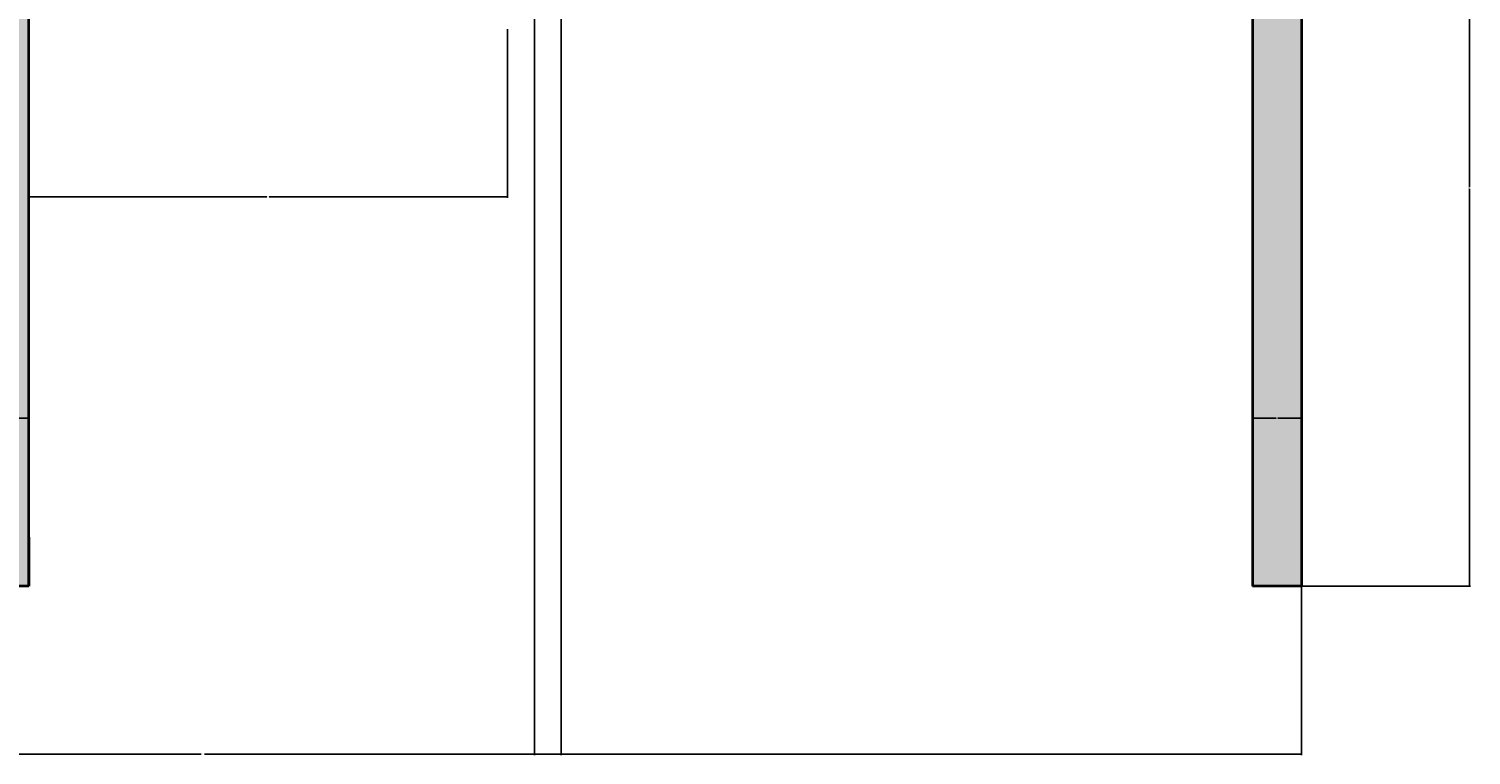
# Model space of a CAD drawing. Units: inches. Extents: x -30 to 437, y -29 to 647.
# Tile 5 of 15: x 172 to 437, y -29 to 105. Entities that reach past the tile are written whole.
import ezdxf

# ---------------------------------------------------------------- set-up
doc = ezdxf.new("R2010")
doc.units = ezdxf.units.IN
doc.header["$MEASUREMENT"] = 0
doc.layers.add('A-ANNO-DIMS', color=2, linetype='Continuous', lineweight=18)
doc.layers.add('A-WALL', color=7, linetype='Continuous', lineweight=35)
doc.layers.add('A-WALL-PATT', color=251, linetype='Continuous', lineweight=13, true_color=0x636466)
doc.styles.get("Standard").update_dxf_attribs({"font": 'arial.ttf'})
doc.dimstyles.get("Standard").update_dxf_attribs({"dimtxt": 0.18, "dimasz": 0.18, "dimexe": 0.18, "dimexo": 0.0625, "dimgap": 0.09, "dimtad": 0, "dimtih": 1, "dimtoh": 1, "dimdec": 4, "dimzin": 0, "dimdsep": 46, "dimtxsty": 'Standard', "dimcen": 0.09, "dimadec": 0, "dimazin": 0, "dimtfac": 1, "dimtdec": 4, "dimtofl": 0, "dimtmove": 0, "dimatfit": 3, "dimfxl": 1, "dimtolj": 1, "dimtzin": 0, "dimarcsym": 0})

# ---------------------------------------------------------------- blocks, each defined once
blk = doc.blocks.new('*D25')
at = {"layer": 'A-ANNO-DIMS', "color": 0, "lineweight": -2, "transparency": 16777216}
for p, q in [((1.67, 1.98), (1.67, -29.03)), ((405.67, 1.98), (405.67, -29.03)), ((1.85, -28.85), (203.38, -28.85)), ((405.49, -28.85), (203.97, -28.85))]:
    blk.add_line(p, q, dxfattribs=at)
at = {"layer": 'A-ANNO-DIMS', "color": 0, "transparency": 16777216}
for points in [[(1.85, -28.82), (1.85, -28.88), (1.67, -28.85)], [(405.49, -28.82), (405.49, -28.88), (405.67, -28.85)]]:
    blk.add_solid(points, dxfattribs=at)
at = {"layer": 'Defpoints', "color": 0, "transparency": 16777216}
for p in [(1.67, 2.05), (405.67, 2.05), (405.67, -28.85)]:
    blk.add_point(p, dxfattribs=at)
at = {"layer": 'A-ANNO-DIMS', "color": 0, "transparency": 16777216, "insert": (203.67, -28.85), "char_height": 0.18, "attachment_point": 5}
blk.add_mtext('\\A1;404', dxfattribs=at)
blk = doc.blocks.new('*D35')
at = {"layer": 'A-ANNO-DIMS', "color": 0, "lineweight": -2, "transparency": 16777216}
for p, q in [((1.67, 2.11), (1.67, 33.13)), ((1.85, 32.95), (86.39, 32.95)), ((171.49, 32.95), (86.95, 32.95)), ((171.67, 2.11), (171.67, 33.13))]:
    blk.add_line(p, q, dxfattribs=at)
at = {"layer": 'A-ANNO-DIMS', "color": 0, "transparency": 16777216}
for points in [[(1.85, 32.98), (1.85, 32.92), (1.67, 32.95)], [(171.49, 32.98), (171.49, 32.92), (171.67, 32.95)]]:
    blk.add_solid(points, dxfattribs=at)
at = {"layer": 'Defpoints', "color": 0, "transparency": 16777216}
for p in [(171.67, 32.95), (1.67, 2.05), (171.67, 2.05)]:
    blk.add_point(p, dxfattribs=at)
at = {"layer": 'A-ANNO-DIMS', "color": 0, "transparency": 16777216, "insert": (86.67, 32.95), "char_height": 0.18, "attachment_point": 5}
blk.add_mtext('\\A1;170', dxfattribs=at)
blk = doc.blocks.new('*D36')
at = {"layer": 'A-ANNO-DIMS', "color": 0, "lineweight": -2, "transparency": 16777216}
for p, q in [((171.67, 104.48), (171.67, 73.47)), ((259.67, 104.48), (259.67, 73.47)), ((171.85, 73.65), (215.45, 73.65)), ((259.49, 73.65), (215.89, 73.65))]:
    blk.add_line(p, q, dxfattribs=at)
at = {"layer": 'A-ANNO-DIMS', "color": 0, "transparency": 16777216}
for points in [[(171.85, 73.68), (171.85, 73.62), (171.67, 73.65)], [(259.49, 73.68), (259.49, 73.62), (259.67, 73.65)]]:
    blk.add_solid(points, dxfattribs=at)
at = {"layer": 'Defpoints', "color": 0, "transparency": 16777216}
for p in [(171.67, 104.55), (259.67, 104.55), (171.67, 73.65)]:
    blk.add_point(p, dxfattribs=at)
at = {"layer": 'A-ANNO-DIMS', "color": 0, "transparency": 16777216, "insert": (215.67, 73.65), "char_height": 0.18, "attachment_point": 5}
blk.add_mtext('\\A1;88', dxfattribs=at)
blk = doc.blocks.new('*D38')
at = {"layer": 'A-ANNO-DIMS', "color": 0, "lineweight": -2, "transparency": 16777216}
for p, q in [((396.67, 2.11), (396.67, 33.13)), ((396.85, 32.95), (401.02, 32.95)), ((405.49, 32.95), (401.32, 32.95)), ((405.67, 2.11), (405.67, 33.13))]:
    blk.add_line(p, q, dxfattribs=at)
at = {"layer": 'A-ANNO-DIMS', "color": 0, "transparency": 16777216}
for points in [[(396.85, 32.98), (396.85, 32.92), (396.67, 32.95)], [(405.49, 32.98), (405.49, 32.92), (405.67, 32.95)]]:
    blk.add_solid(points, dxfattribs=at)
at = {"layer": 'Defpoints', "color": 0, "transparency": 16777216}
for p in [(405.67, 32.95), (396.67, 2.05), (405.67, 2.05)]:
    blk.add_point(p, dxfattribs=at)
at = {"layer": 'A-ANNO-DIMS', "color": 0, "transparency": 16777216, "insert": (401.17, 32.95), "char_height": 0.18, "attachment_point": 5}
blk.add_mtext('\\A1;9', dxfattribs=at)
blk = doc.blocks.new('*D39')
at = {"layer": 'A-ANNO-DIMS', "color": 0, "lineweight": -2, "transparency": 16777216}
for p, q in [((396.74, 148.55), (436.75, 148.55)), ((436.57, 148.37), (436.57, 75.48)), ((436.57, 2.23), (436.57, 75.12)), ((396.74, 2.05), (436.75, 2.05))]:
    blk.add_line(p, q, dxfattribs=at)
at = {"layer": 'A-ANNO-DIMS', "color": 0, "transparency": 16777216}
for points in [[(436.54, 148.37), (436.6, 148.37), (436.57, 148.55)], [(436.54, 2.23), (436.6, 2.23), (436.57, 2.05)]]:
    blk.add_solid(points, dxfattribs=at)
at = {"layer": 'Defpoints', "color": 0, "transparency": 16777216}
for p in [(396.67, 148.55), (436.57, 148.55), (396.67, 2.05)]:
    blk.add_point(p, dxfattribs=at)
at = {"layer": 'A-ANNO-DIMS', "color": 0, "transparency": 16777216, "insert": (436.57, 75.3), "char_height": 0.18, "attachment_point": 5}
blk.add_mtext('\\A1;146.5', dxfattribs=at)
blk = doc.blocks.new('*D56')
at = {"layer": 'A-ANNO-DIMS', "color": 0, "lineweight": -2, "transparency": 16777216}
for p, q in [((269.54, 160.3), (269.54, -29.03)), ((264.67, 153.48), (264.67, -29.03)), ((264.85, -28.85), (266.78, -28.85)), ((269.36, -28.85), (267.44, -28.85))]:
    blk.add_line(p, q, dxfattribs=at)
at = {"layer": 'A-ANNO-DIMS', "color": 0, "transparency": 16777216}
for points in [[(264.85, -28.82), (264.85, -28.88), (264.67, -28.85)], [(269.36, -28.82), (269.36, -28.88), (269.54, -28.85)]]:
    blk.add_solid(points, dxfattribs=at)
at = {"layer": 'Defpoints', "color": 0, "transparency": 16777216}
for p in [(269.54, 160.37), (264.67, 153.55), (269.54, -28.85)]:
    blk.add_point(p, dxfattribs=at)
at = {"layer": 'A-ANNO-DIMS', "color": 0, "transparency": 16777216, "insert": (267.11, -28.85), "char_height": 0.18, "attachment_point": 5}
blk.add_mtext('\\A1;4.87', dxfattribs=at)

msp = doc.modelspace()

# ---------------------------------------------------------------- hatches: boundary and pattern name
at = {"layer": 'A-WALL-PATT'}
h = msp.add_hatch(color=256, dxfattribs=at)
h.dxf.hatch_style = 1
h.paths.add_polyline_path([(393.6054, 183.2352), (369.6054, 183.2352), (369.6054, 213.2352), (393.6054, 213.2352), (393.6054, 207.2352), (394.6054, 207.2352), (394.6054, 211.2352), (395.6054, 211.2352), (395.6054, 185.2352), (394.6054, 185.2352), (394.6054, 189.2352), (393.6054, 189.2352)], flags=0)
h.paths.add_polyline_path([(384.6054, 189.2352, -1), (390.6054, 189.2352, -1)], flags=0)
h.paths.add_polyline_path([(385.6054, 189.2352, -1), (389.6054, 189.2352, -1)], flags=0)
h.paths.add_polyline_path([(374.6054, 189.2352, -1), (382.6054, 189.2352, -1)], flags=0)
h.paths.add_polyline_path([(386.6054, 189.2352, -1), (388.6054, 189.2352, -1)], flags=0)
h.paths.add_polyline_path([(375.6054, 189.2352, -1), (381.6054, 189.2352, -1)], flags=0)
h.paths.add_polyline_path([(376.6054, 189.2352, -1), (380.6054, 189.2352, -1)], flags=0)
h.paths.add_polyline_path([(377.6054, 189.2352, -1), (379.6054, 189.2352, -1)], flags=0)
h.paths.add_polyline_path([(390.6054, 195.2352), (374.6054, 195.2352), (374.6054, 201.2352), (390.6054, 201.2352)], flags=0)
h.paths.add_polyline_path([(389.6054, 196.2352), (375.6054, 196.2352), (375.6054, 200.2352), (389.6054, 200.2352)], flags=0)
h.paths.add_polyline_path([(383.6054, 207.2352, -1), (391.6054, 207.2352, -1)], flags=0)
h.paths.add_polyline_path([(384.6054, 207.2352, -1), (390.6054, 207.2352, -1)], flags=0)
h.paths.add_polyline_path([(385.6054, 207.2352, -1), (389.6054, 207.2352, -1)], flags=0)
h.paths.add_polyline_path([(386.6054, 207.2352, -1), (388.6054, 207.2352, -1)], flags=0)
h.paths.add_polyline_path([(375.6054, 207.2352, -1), (381.6054, 207.2352, -1)], flags=0)
h.paths.add_polyline_path([(376.6054, 207.2352, -1), (380.6054, 207.2352, -1)], flags=0)
h.paths.add_polyline_path([(377.6054, 207.2352, -1), (379.6054, 207.2352, -1)], flags=0)
h.paths.add_polyline_path([(305.5437, 160.3663, -0.41421356), (304.0437, 158.8663), (271.0437, 158.8663, -0.41421356), (269.5437, 160.3663), (269.5437, 178.3663, -0.41421356), (271.0437, 179.8663), (304.0437, 179.8663, -0.41421356), (305.5437, 178.3663)], flags=0)
h.paths.add_polyline_path([(304.0437, 165.3663, -0.41421356), (303.0437, 164.3663), (289.2937, 164.3663, -0.41421356), (288.2937, 165.3663), (288.2937, 177.3663, -0.41421356), (289.2937, 178.3663), (303.0437, 178.3663, -0.41421356), (304.0437, 177.3663)], flags=0)
h.paths.add_polyline_path([(296.5437, 171.3663, -1), (295.5437, 171.3663, -1)], flags=0)
h.paths.add_polyline_path([(286.7937, 165.3663, -0.41421356), (285.7937, 164.3663), (272.0437, 164.3663, -0.41421356), (271.0437, 165.3663), (271.0437, 177.3663, -0.41421356), (272.0437, 178.3663), (285.7937, 178.3663, -0.41421356), (286.7937, 177.3663)], flags=0)
h.paths.add_polyline_path([(279.5437, 171.3663, -1), (278.5437, 171.3663, -1)], flags=0)
h.paths.add_polyline_path([(360.6737, 290.5474), (360.6737, 300.5474), (396.6737, 300.5474), (396.6737, 290.5474)], flags=0)
h.paths.add_polyline_path([(259.6737, 124.5474), (259.6737, 114.5474), (171.6737, 114.5474), (171.6737, 124.5474)], flags=0)
h.paths.add_polyline_path([(288.0737, 215.3705), (286.7097, 214.583), (268.7097, 245.7599), (270.0737, 246.5474)], flags=0)
h.paths.add_polyline_path([(259.6737, 168.5474), (256.6737, 168.5474), (256.6737, 173.5474), (256.6737, 179.0224), (255.8753, 177.6395), (224.2956, 195.872, 0.12053744), (220.1737, 179.0224, 0.12053744), (216.0518, 195.872), (184.4721, 177.6395), (183.6737, 179.0224), (215.2836, 197.2724), (216.0821, 195.8895), (216.0518, 195.872, -0.12053744), (220.1737, 179.0224, -0.12053744), (224.2956, 195.872), (224.2653, 195.8895), (225.0638, 197.2724), (256.6737, 179.0224), (256.6737, 173.5474), (259.6737, 173.5474)], flags=0)
h.paths.add_polyline_path([(386.7943, 325.4601), (372.6871, 325.4601), (372.6871, 339.5673), (386.7943, 339.5673)], flags=0)
h.paths.add_polyline_path([(359.5875, 343.7429), (357.7905, 343.7429), (357.7905, 327.9179), (359.3933, 327.9179, 0.41420885), (361.5302, 330.0549), (361.5302, 341.8434, 0.41436161)], flags=0)
h.paths.add_polyline_path([(341.7887, 323.1235, -0.11921667), (340.7839, 323.1235)], flags=0)
h.paths.add_polyline_path([(379.6332, 328.8632), (379.6332, 332.2699), (376.0992, 332.2699, 0.39427733)], flags=0)
h.paths.add_polyline_path([(375.5299, 332.459, -1), (383.8511, 332.459, -1)], flags=0)
h.paths.add_polyline_path([(388.9363, 344.7425), (372.5309, 344.7425, -0.41421356), (370.394, 346.8794), (370.394, 347.5594, -0.39085173), (372.3472, 349.7005, -0.43951011), (370.394, 351.4933), (370.394, 365.1894, -0.40305452), (372.2191, 367.1298, -0.41839453), (370.394, 368.9291), (370.394, 382.6251, -0.40885826), (372.2519, 384.5722, -0.42377324), (370.394, 386.3707), (370.394, 400.0667, -0.38660687), (372.1327, 402.0094), (372.531, 402.0094, -0.41421834), (370.394, 404.1464), (370.394, 404.7778, -0.41420891), (372.5309, 406.9147), (388.9363, 406.9147, -0.41421821), (391.0733, 404.7778), (391.0733, 346.8794, -0.41421356)], flags=0)
edge = h.paths.add_edge_path(flags=0)
edge.add_spline(control_points=[(349.3585, 363.204), (349.0859, 363.204), (348.8133, 363.2227), (348.2712, 363.2973), (348.0016, 363.3531), (347.3533, 363.5328), (346.9776, 363.6755), (346.2445, 364.0308), (345.887, 364.2432), (345.1953, 364.7329), (344.8611, 365.0101), (344.2197, 365.6237), (343.9125, 365.9603), (343.211, 366.8336), (342.8313, 367.3965), (342.1401, 368.6117), (341.8286, 369.2641), (341.2807, 370.64), (341.0443, 371.3636), (340.6522, 372.8619), (340.4964, 373.6367), (340.2695, 375.2158), (340.1983, 376.0203), (340.142, 377.6365), (340.157, 378.4483), (340.2729, 380.0567), (340.3738, 380.8533), (340.6589, 382.4093), (340.8432, 383.1686), (341.2906, 384.629), (341.5538, 385.3301), (342.1531, 386.6544), (342.4891, 387.2776), (343.2266, 388.4288), (343.6281, 388.9567), (344.4879, 389.9012), (344.9463, 390.3178), (345.7981, 390.9428), (346.182, 391.1771), (346.9712, 391.5648), (347.3766, 391.7182), (348.2004, 391.9387), (348.6189, 392.0058), (349.4588, 392.0508), (349.8801, 392.0288), (350.7146, 391.8966), (351.1278, 391.7865), (351.9366, 391.4822), (352.3323, 391.2882), (353.0989, 390.8223), (353.4699, 390.5504), (354.1819, 389.9355), (354.5229, 389.5924), (355.1706, 388.8418), (355.4772, 388.4343), (356.1315, 387.4422), (356.4671, 386.8397), (357.0692, 385.5581), (357.3356, 384.879), (357.7933, 383.4624), (357.9846, 382.725), (358.2875, 381.2112), (358.3992, 380.4349), (358.5404, 378.8643), (358.5699, 378.0699), (358.546, 376.4841), (358.4926, 375.6928), (358.3042, 374.1343), (358.1692, 373.3672), (357.8207, 371.8774), (357.6072, 371.1549), (357.1067, 369.7735), (356.8196, 369.1148), (356.1782, 367.8787), (355.8238, 367.3013), (355.0551, 366.244), (354.6408, 365.7641), (353.7607, 364.9161), (353.2948, 364.5481), (352.445, 364.0149), (352.0701, 363.822), (351.3034, 363.5117), (350.9116, 363.3943), (350.1325, 363.2418), (349.7455, 363.204), (349.3585, 363.204)], knot_values=[3.14159265, 3.14159265, 3.14159265, 3.14159265, 3.22691715, 3.22691715, 3.31224165, 3.31224165, 3.43426671, 3.43426671, 3.55629177, 3.55629177, 3.67831683, 3.67831683, 3.8003419, 3.8003419, 3.97157384, 3.97157384, 4.14280577, 4.14280577, 4.31403771, 4.31403771, 4.48526965, 4.48526965, 4.65650159, 4.65650159, 4.82773353, 4.82773353, 4.99896547, 4.99896547, 5.1701974, 5.1701974, 5.34142934, 5.34142934, 5.51266128, 5.51266128, 5.68389322, 5.68389322, 5.85512516, 5.85512516, 5.98669107, 5.98669107, 6.11825699, 6.11825699, 6.24982291, 6.24982291, 6.38138882, 6.38138882, 6.51295474, 6.51295474, 6.64452065, 6.64452065, 6.77608657, 6.77608657, 6.90765249, 6.90765249, 7.0392184, 7.0392184, 7.20701563, 7.20701563, 7.37481286, 7.37481286, 7.54261009, 7.54261009, 7.71040732, 7.71040732, 7.87820455, 7.87820455, 8.04600178, 8.04600178, 8.21379901, 8.21379901, 8.38159624, 8.38159624, 8.54939347, 8.54939347, 8.7171907, 8.7171907, 8.88498794, 8.88498794, 9.05278517, 9.05278517, 9.17820699, 9.17820699, 9.30362881, 9.30362881, 9.42477796, 9.42477796, 9.42477796, 9.42477796], degree=3, periodic=0)
edge.add_line((341.1696, 384.3006), (341.2012, 384.2808))
edge = h.paths.add_edge_path(flags=0)
edge.add_line((344.3353, 388.7801), (344.317, 388.7915))
edge.add_ellipse((349.3585, 377.6204), major_axis=(0, -13.7895), ratio=0.62186025, start_angle=-244.867444, end_angle=-124.769923)
h.paths.add_polyline_path([(163.6737, 163.1474), (132.4968, 145.1474), (131.7093, 146.5114), (162.8862, 164.5114)], flags=0)
h.paths.add_polyline_path([(366.4355, 409.0896, -0.41423669), (364.2985, 406.9525, -0.4913499), (361.5302, 408.8973), (361.5302, 420.6405, 0.41421356), (359.3932, 422.7775), (357.7905, 422.7775), (357.7905, 406.9525), (359.6317, 406.9525, 0.42741026), (361.5332, 408.9757, 0.39869469), (363.6672, 406.9525, 0.51958103), (366.4355, 409.0895)], flags=0)
h.paths.add_polyline_path([(386.7943, 410.9671), (372.6871, 410.9671), (372.6871, 425.0742), (386.7943, 425.0742)], flags=0)
h.paths.add_polyline_path([(379.6332, 414.3701), (379.6332, 417.7768), (376.0992, 417.7768, 0.39427733)], flags=0)
h.paths.add_polyline_path([(375.5299, 417.966, -1), (383.8511, 417.966, -1)], flags=0)
h.paths.add_polyline_path([(150.0377, 351.583), (148.6737, 352.3705), (166.6737, 383.5474), (168.0377, 382.7599)], flags=0)
h.paths.add_polyline_path([(91.6737, 234.1974), (66.559, 219.6974), (65.9246, 220.7962), (91.0393, 235.2962)], flags=0)
h.paths.add_polyline_path([(255.4612, 443.5834), (254.6737, 444.9474), (285.8506, 462.9474), (286.6381, 461.5834)], flags=0)
h.paths.add_polyline_path([(176.2737, 394.5474), (158.2737, 425.7243), (159.6377, 426.5118), (177.6377, 395.3349)], flags=0)
h.paths.add_polyline_path([(243.6737, 439.5474), (243.0393, 438.4486), (217.9246, 452.9486), (218.559, 454.0474)], flags=0)
h.paths.add_polyline_path([(38.1264, 269.8429), (40.2408, 269.8429), (40.2408, 270.3508), (38.1264, 270.3508)], flags=0)
h.paths.add_polyline_path([(75.7157, 289.9439), (40.2408, 289.9439), (38.1264, 289.6524), (40.2408, 289.6524)], flags=0)
h.paths.add_polyline_path([(75.7157, 270.0846), (77.6447, 270.0846), (77.6697, 270.1626), (75.7175, 270.1626)], flags=0)
h.paths.add_polyline_path([(80.5373, 293.3002), (33.0467, 293.3002), (13.5054, 293.3002), (13.5054, 351.9244), (29.7898, 351.9244), (80.5373, 351.9244)], flags=0)
h.paths.add_polyline_path([(46.0261, 212.466, -0.50131678), (27.1651, 207.5106), (21.165, 209.5107), (21.165, 206.5107), (22.665, 206.5107), (22.665, 203.5107), (21.165, 203.5107), (21.165, 203.0107), (13.165, 203.0107), (13.165, 224.0107), (21.165, 224.0107), (21.165, 217.5107), (27.1649, 219.5106, -0.50132349), (46.0261, 214.5554, -0.13289091)], flags=0)
h.paths.add_polyline_path([(44.688, 211.8666, -0.48007965), (27.165, 209.5107), (27.165, 217.5107, -0.4800795), (44.688, 215.1547, -0.21500378)], flags=0)
h.paths.add_polyline_path([(19.415, 204.0107), (15.165, 204.0107, -0.41421356), (14.165, 204.7607), (14.165, 222.0107, -0.41421356), (14.915, 223.0107), (19.165, 223.0107, -0.41421356), (20.165, 222.2607), (20.165, 205.0107, -0.41421356)], flags=0)
h.paths.add_polyline_path([(32.7608, 269.0719), (31.8439, 269.0719), (31.8439, 268.6134), (13.5054, 268.6134), (13.5054, 291.5366), (31.8439, 291.5366), (32.7608, 291.0781), (32.7608, 280.9919, -1), (32.7608, 279.1581)], flags=0)
h.paths.add_polyline_path([(40.2408, 360.1436), (38.1264, 360.1436), (38.1264, 359.6357), (40.2408, 359.6357)], flags=0)
h.paths.add_polyline_path([(75.7157, 355.2807), (40.2408, 355.2807), (38.1264, 355.5722), (40.2408, 355.5722), (40.2408, 355.2807), (75.7157, 355.2807), (75.7157, 375.5982), (40.2408, 375.5982), (38.1264, 375.3817), (40.2408, 375.3817), (40.2408, 375.5982), (75.7157, 375.5982), (77.9733, 375.062), (75.7175, 375.062), (75.7175, 374.554)], flags=0)
h.paths.add_polyline_path([(42.8174, 299.814, 0.13867074), (34.1602, 294.603), (14.8081, 294.603), (14.8081, 350.6216), (29.8539, 350.6216, 0.09822056)], flags=0)
h.paths.add_polyline_path([(15.8636, 276.7781, -0.30640166), (20.3757, 283.4499), (20.3483, 290.6726), (31.4014, 290.7146), (31.4309, 282.9124), (26.8287, 282.895, -0.26006276), (30.241, 276.7781, -1)], flags=0)
h.paths.add_polyline_path([(26.1332, 276.7781), (23.0523, 273.6972), (19.9714, 276.7781), (23.0523, 279.8589), (23.0523, 283.9209), (21.3493, 283.9145), (20.7006, 283.5219), (20.6907, 286.1226), (23.2914, 286.1325), (25.8936, 285.7522), (27.1939, 285.7572), (28.4928, 286.1522), (31.0935, 286.1621), (31.0918, 286.6172), (25.6303, 286.5965), (25.616, 290.3675), (31.0775, 290.3882), (31.0918, 286.6172), (31.1034, 283.5614), (28.5027, 283.5515), (25.9005, 283.9317), (23.0523, 283.9209), (23.0523, 279.8589)], flags=0)
h.paths.add_polyline_path([(24.0793, 276.7781, -1), (22.0253, 276.7781, -1)], flags=0)
h.paths.add_polyline_path([(35.7687, 302.2895, -0.41421356), (35.2283, 301.2726), (22.2164, 297.2909, -0.41421356), (21.1995, 297.8313), (15.7317, 315.6996, -0.41421356), (16.2721, 316.7165), (18.8554, 317.507), (15.3721, 328.8904, -0.41421356), (15.9125, 329.9073), (28.9244, 333.889, -0.41421356), (29.9414, 333.3486), (35.4091, 315.4802, -0.41421356), (34.8687, 314.4633), (32.2854, 313.6728)], flags=0)
h.paths.add_polyline_path([(361.3728, 532.6207), (302.7487, 532.6207), (302.7487, 580.1113), (302.7487, 599.6527), (361.3728, 599.6527), (361.3728, 583.3682)], flags=0)
h.paths.add_polyline_path([(370.1, 575.0316), (370.1, 572.9172), (370.6079, 572.9172), (370.6079, 575.0316)], flags=0)
h.paths.add_polyline_path([(385.0466, 537.4423), (385.0466, 572.9172), (384.8302, 575.0316), (384.8302, 572.9172)], flags=0)
h.paths.add_polyline_path([(384.5104, 535.3262), (384.5104, 537.4406), (384.0025, 537.4406), (364.7291, 537.4423), (364.7291, 572.9172), (365.0206, 575.0316), (365.0206, 572.9172), (364.7291, 572.9172), (364.7291, 537.4423), (384.5884, 537.4423), (384.5884, 535.5133)], flags=0)
h.paths.add_polyline_path([(384.5884, 535.5133), (383.4945, 535.164), (383.4945, 537.4406), (382.9866, 535.3262), (382.9866, 537.4406), (383.4945, 535.3262), (383.4945, 537.4406), (384.5884, 537.4406)], flags=0)
h.paths.add_polyline_path([(23.874, 286.8174), (21.0132, 286.8065), (21.0004, 290.1875), (23.8612, 290.1983)], flags=0)
h.paths.add_polyline_path([(242.9824, 511.1667), (234.9824, 511.1667), (234.9824, 517.6667), (228.9825, 515.6667, -0.50132349), (210.1213, 520.622, -0.13289091), (210.1213, 522.7114, -0.50131678), (228.9823, 527.6667), (234.9824, 525.6667), (234.9824, 528.6667), (233.4824, 528.6667), (233.4824, 531.6667), (234.9824, 531.6667), (234.9824, 532.1667), (242.9824, 532.1667)], flags=0)
h.paths.add_polyline_path([(236.9824, 512.1667, -0.41421356), (235.9824, 512.9167), (235.9824, 530.1667, -0.41421356), (236.7324, 531.1667), (240.9824, 531.1667, -0.41421356), (241.9824, 530.4167), (241.9824, 513.1667, -0.41421356), (241.2324, 512.1667)], flags=0)
h.paths.add_polyline_path([(279.533, 537.4423), (279.533, 535.5133), (279.6111, 535.4884), (279.6111, 537.4406)], flags=0)
h.paths.add_polyline_path([(279.2913, 575.0316), (279.2913, 572.9172), (279.7992, 572.9172), (279.7992, 575.0316)], flags=0)
h.paths.add_polyline_path([(211.4594, 520.0227, -0.21500378), (211.4594, 523.3107, -0.48007965), (228.9824, 525.6667), (228.9824, 517.6667, -0.4800795)], flags=0)
h.paths.add_polyline_path([(32.7627, 354.1465), (31.8457, 354.1465), (31.8457, 353.688), (13.5054, 353.688), (13.5054, 376.6134), (31.8457, 376.6134), (32.7627, 376.1549), (32.7627, 366.0677, -1), (32.7627, 364.2337)], flags=0)
h.paths.add_polyline_path([(15.9446, 365.1507, -1), (30.3234, 365.1507, -1)], flags=0)
h.paths.add_polyline_path([(41.213, 428.467), (43.3274, 428.467), (43.3274, 428.9749), (41.213, 428.9749)], flags=0)
h.paths.add_polyline_path([(78.8022, 448.568), (43.3274, 448.568), (41.213, 448.2765), (43.3274, 448.2765)], flags=0)
h.paths.add_polyline_path([(78.8022, 428.7087), (80.7313, 428.7087), (80.7562, 428.7868), (78.804, 428.7868)], flags=0)
h.paths.add_polyline_path([(26.2152, 365.1507), (23.134, 362.0696), (20.0529, 365.1507), (23.134, 368.2319)], flags=0)
h.paths.add_polyline_path([(24.1611, 365.1507, -1), (22.107, 365.1507, -1)], flags=0)
h.paths.add_polyline_path([(309.2625, 570.3406, 0.13867074), (304.0514, 578.9978), (304.0514, 598.3499), (360.07, 598.3499), (360.07, 583.3041, 0.09822056)], flags=0)
h.paths.add_polyline_path([(246.6737, 552.5474), (129.6737, 552.5474), (129.6737, 606.5474), (246.6737, 606.5474)], flags=16)
h.paths.add_polyline_path([(373.6822, 580.3953), (363.595, 580.3953), (363.595, 581.3123), (363.1365, 581.3123), (363.1365, 599.6527), (386.0619, 599.6527), (386.0619, 581.3123), (385.6034, 580.3953), (375.5162, 580.3953, -1)], flags=0)
h.paths.add_polyline_path([(83.6239, 451.9244), (36.1333, 451.9244), (16.5919, 451.9244), (16.5919, 510.5485), (32.8764, 510.5485), (83.6239, 510.5485)], flags=0)
h.paths.add_polyline_path([(367.4098, 590.024, -1), (381.7886, 590.024, -1)], flags=0)
h.paths.add_polyline_path([(374.5992, 586.9428), (371.518, 590.024), (374.5992, 593.1052), (377.6803, 590.024)], flags=0)
h.paths.add_polyline_path([(373.5721, 590.024, -1), (375.6262, 590.024, -1)], flags=0)
h.paths.add_polyline_path([(324.9287, 577.7489, -0.41421356), (323.9118, 578.2893), (323.1212, 580.8726), (311.7379, 577.3893, -0.41421356), (310.721, 577.9297), (306.7393, 590.9416, -0.41421356), (307.2797, 591.9585), (325.1481, 597.4263, -0.41421356), (326.165, 596.8859), (326.9555, 594.3026), (338.3388, 597.7859, -0.41421356), (339.3557, 597.2455), (343.3374, 584.2336, -0.41421356), (342.797, 583.2167)], flags=0)
h.paths.add_polyline_path([(300.5265, 580.3972), (290.4404, 580.3972, -1), (288.6065, 580.3972), (278.5203, 580.3972), (278.5203, 581.3142), (278.0619, 581.3142), (278.0619, 599.6527), (300.985, 599.6527), (300.985, 581.3142)], flags=0)
h.paths.add_polyline_path([(300.163, 581.7567), (292.3609, 581.7271), (292.3434, 586.3294, -0.75567924), (279.0378, 590.1057, -0.82536731), (292.8983, 592.7823), (300.1211, 592.8097)], flags=0)
h.paths.add_polyline_path([(299.8367, 582.0805), (296.0656, 582.0662), (293.0098, 582.0546), (292.9999, 584.6553), (293.3802, 587.2575), (293.3694, 590.1057), (289.3074, 590.1057), (286.2265, 587.0248), (283.1456, 590.1057), (286.2265, 593.1866), (289.3074, 590.1057), (293.3694, 590.1057), (293.3629, 591.8088), (292.9703, 592.4575), (295.5711, 592.4673), (295.5809, 589.8666), (295.2007, 587.2644), (295.2056, 585.9641), (295.6006, 584.6652), (295.6105, 582.0645), (296.0656, 582.0662), (296.0449, 587.5277), (299.8159, 587.542)], flags=0)
h.paths.add_polyline_path([(285.1995, 590.1057, -1), (287.2535, 590.1057, -1)], flags=0)
h.paths.add_polyline_path([(299.6467, 589.2969), (296.2658, 589.284), (296.255, 592.1448), (299.6359, 592.1576)], flags=0)
h.paths.add_polyline_path([(35.8473, 427.696), (34.9304, 427.696), (34.9304, 427.2376), (16.5919, 427.2376), (16.5919, 450.1607), (34.9304, 450.1607), (35.8473, 449.7022), (35.8473, 439.6161, -1), (35.8473, 437.7822)], flags=0)
h.paths.add_polyline_path([(18.9502, 435.4022, -0.30640166), (23.4623, 442.074), (23.4349, 449.2968), (34.4879, 449.3387), (34.5175, 441.5366), (29.9152, 441.5191, -0.26006276), (33.3275, 435.4022, -1)], flags=0)
h.paths.add_polyline_path([(29.2197, 435.4022), (26.1389, 432.3213), (23.058, 435.4022), (26.1389, 438.4831), (26.1389, 442.5451), (24.4358, 442.5386), (23.7871, 442.1461), (23.7772, 444.7468), (26.378, 444.7566), (28.9801, 444.3764), (30.2805, 444.3813), (31.5794, 444.7764), (34.1801, 444.7862), (34.1784, 445.2413), (28.7169, 445.2206), (28.7026, 448.9917), (34.164, 449.0124), (34.1784, 445.2413), (34.1899, 442.1855), (31.5892, 442.1756), (28.987, 442.5559), (26.1389, 442.5451), (26.1389, 438.4831)], flags=0)
h.paths.add_polyline_path([(27.1658, 435.4022, -1), (25.1119, 435.4022, -1)], flags=0)
h.paths.add_polyline_path([(45.904, 458.4382, 0.13867074), (37.2467, 453.2271), (17.8947, 453.2271), (17.8947, 509.2457), (32.9405, 509.2457, 0.09822056)], flags=0)
h.paths.add_polyline_path([(26.9605, 445.4415), (24.0997, 445.4307), (24.0869, 448.8116), (26.9477, 448.8225)], flags=0)
h.paths.add_polyline_path([(38.3149, 459.8967), (25.3029, 455.915, -0.41421356), (24.286, 456.4554), (18.8183, 474.3238, -0.41421356), (19.3586, 475.3407), (21.942, 476.1312), (18.4587, 487.5145, -0.41421356), (18.999, 488.5314), (32.011, 492.5131, -0.41421356), (33.0279, 491.9727), (38.4957, 474.1044, -0.41421356), (37.9553, 473.0875), (35.3719, 472.297), (38.8553, 460.9136, -0.41421356)], flags=0)
h.paths.add_polyline_path([(43.3274, 518.7678), (41.213, 518.7678), (41.213, 518.2598), (43.3274, 518.2598)], flags=0)
h.paths.add_polyline_path([(78.8022, 513.9049), (43.3274, 513.9049), (41.213, 514.1964), (43.3274, 514.1964), (43.3274, 513.9049), (78.8022, 513.9049), (78.8022, 534.2223), (43.3274, 534.2223), (41.213, 534.0059), (43.3274, 534.0059), (43.3274, 534.2223), (78.8022, 534.2223), (81.0599, 533.6861), (78.804, 533.6861), (78.804, 533.1782)], flags=0)
h.paths.add_polyline_path([(121.6737, 556.8974), (121.0393, 555.7986), (95.9246, 570.2986), (96.559, 571.3974)], flags=0)
h.paths.add_polyline_path([(35.8493, 512.7707), (34.9322, 512.7707), (34.9322, 512.3122), (16.5919, 512.3122), (16.5919, 535.2376), (34.9322, 535.2376), (35.8493, 534.7791), (35.8493, 524.6919, -1), (35.8493, 522.8579)], flags=0)
h.paths.add_polyline_path([(19.0312, 523.7749, -1), (33.41, 523.7749, -1)], flags=0)
h.paths.add_polyline_path([(26.2206, 520.6937), (23.1394, 523.7749), (26.2206, 526.8561), (29.3018, 523.7749)], flags=0)
h.paths.add_polyline_path([(25.1935, 523.7749, -1), (27.2476, 523.7749, -1)], flags=0)
h.paths.add_polyline_path([(28.4381, 586.0173), (22.438, 588.0173), (22.438, 585.0173), (23.938, 585.0173), (23.938, 582.0173), (22.438, 582.0173), (22.438, 581.5173), (14.438, 581.5173), (14.438, 602.5173), (22.438, 602.5173), (22.438, 596.0173), (28.4379, 598.0173, -0.50132349), (47.2992, 593.062, -0.13289091), (47.2992, 590.9726, -0.50131678)], flags=0)
h.paths.add_polyline_path([(28.438, 588.0174), (28.438, 596.0173, -0.4800795), (45.961, 593.6614, -0.21500378), (45.961, 590.3733, -0.48007965)], flags=0)
h.paths.add_polyline_path([(20.688, 582.5173), (16.438, 582.5173, -0.41421356), (15.438, 583.2673), (15.438, 600.5173, -0.41421356), (16.188, 601.5173), (20.438, 601.5173, -0.41421356), (21.438, 600.7673), (21.438, 583.5173, -0.41421356)], flags=0)
h.paths.add_polyline_path([(171.6737, 2.0474), (171.6737, 104.5474), (259.6737, 104.5474), (259.6737, 148.5474), (396.6737, 148.5474), (396.6737, 2.0474), (405.6737, 2.0474), (405.6737, 615.5474), (1.6737, 615.5474), (1.6737, 2.0474)])
h.paths.add_polyline_path([(171.6737, 104.5474), (259.6737, 104.5474), (259.6737, 210.5474), (264.6737, 210.5474), (264.6737, 153.5474), (396.6737, 153.5474), (396.6737, 249.5474), (264.6737, 249.5474), (264.6737, 246.5474), (259.6737, 246.5474), (259.6737, 254.5474), (396.6737, 254.5474), (396.6737, 434.5474), (290.6737, 434.5474), (290.6737, 439.5474), (396.6737, 439.5474), (396.6737, 606.5474), (251.6737, 606.5474), (251.6737, 439.5474), (254.6737, 439.5474), (254.6737, 434.5474), (243.6737, 434.5474), (243.6737, 439.5474), (246.6737, 439.5474), (246.6737, 547.5474), (186.6737, 547.5474), (186.6737, 439.5474), (214.6737, 439.5474), (214.6737, 434.5474), (186.6737, 434.5474), (186.6737, 430.5474), (181.6737, 430.5474), (181.6737, 547.5474), (121.6737, 547.5474), (121.6737, 552.5474), (124.6737, 552.5474), (124.6737, 606.5474), (10.6737, 606.5474), (10.6737, 552.5474), (92.6737, 552.5474), (92.6737, 547.5474), (10.6737, 547.5474), (10.6737, 391.5474), (181.6737, 391.5474), (181.6737, 394.5474), (186.6737, 394.5474), (186.6737, 386.5474), (171.6737, 386.5474), (171.6737, 383.5474), (166.6737, 383.5474), (166.6737, 386.5474), (10.6737, 386.5474), (10.6737, 238.5474), (62.6737, 238.5474), (62.6737, 233.5474), (10.6737, 233.5474), (10.6737, 173.5474), (94.6737, 173.5474), (94.6737, 233.5474), (91.6737, 233.5474), (91.6737, 238.5474), (166.6737, 238.5474), (166.6737, 347.5474), (171.6737, 347.5474), (171.6737, 233.5474), (99.6737, 233.5474), (99.6737, 173.5474), (127.6737, 173.5474), (127.6737, 168.5474), (10.6737, 168.5474), (10.6737, 11.0474), (166.6737, 11.0474), (166.6737, 168.5474), (163.6737, 168.5474), (163.6737, 173.5474), (183.6737, 173.5474), (183.6737, 168.5474), (171.6737, 168.5474)])

# ---------------------------------------------------------------- linework, layer by layer
at = {"layer": 'A-WALL'}
for p, q in [((171.6737, 2.0474), (171.6737, 168.5474)), ((396.6737, 148.5474), (396.6737, 11.0474)), ((171.6737, 11.0474), (171.6737, 2.0474)), ((171.6737, 11.0474), (171.6737, 2.0474)), ((396.6737, 11.0474), (396.6737, 2.0474))]:
    msp.add_line(p, q, dxfattribs=at)
msp.add_lwpolyline([(171.6737, 2.0474), (1.6737, 2.0474), (1.6737, 615.5474), (405.6737, 615.5474), (405.6737, 2.0474), (396.6737, 2.0474)], dxfattribs=at)

# ---------------------------------------------------------------- dimensions: what is measured, and where the dimension line sits
at = {"layer": 'A-ANNO-DIMS'}
for base, p1, p2, override, picture, middle in [((269.5437, -28.8526), (264.6737, 153.5474), (269.5437, 160.3663), {"dimdec": 2, "dimlfac": 1, "dimrnd": 0, "dimzin": 0, "dimdsep": 46, "dimlunit": 2}, '*D56', (267.1087, -28.8526)), ((171.6737, 32.9474), (1.6737, 2.0474), (171.6737, 2.0474), {"dimdec": 0, "dimlfac": 1, "dimrnd": 0, "dimzin": 0, "dimdsep": 46, "dimlunit": 2}, '*D35', (86.6737, 32.9474)), ((405.6737, 32.9474), (396.6737, 2.0474), (405.6737, 2.0474), {"dimdec": 0, "dimlfac": 1, "dimrnd": 0, "dimzin": 0, "dimdsep": 46, "dimlunit": 2}, '*D38', (401.1737, 32.9474)), ((405.6737, -28.8526), (1.6737, 2.0474), (405.6737, 2.0474), {"dimdec": 0, "dimlfac": 1, "dimrnd": 0, "dimzin": 0, "dimdsep": 46, "dimlunit": 2}, '*D25', (203.6737, -28.8526))]:
    dim = msp.add_linear_dim(base=base, p1=p1, p2=p2, dimstyle='Standard', override=override, dxfattribs=at)
    dim.commit()
    dim.dimension.update_dxf_attribs({"geometry": picture, "text_midpoint": middle})
for base, p1, p2, angle, override, picture, middle in [((436.5737, 148.5474), (396.6737, 2.0474), (396.6737, 148.5474), 90, {"dimdec": 1, "dimlfac": 1, "dimrnd": 0, "dimzin": 0, "dimdsep": 46, "dimlunit": 2}, '*D39', (436.5737, 75.2974)), ((171.6737, 73.6474), (259.6737, 104.5474), (171.6737, 104.5474), 180, {"dimdec": 0, "dimlfac": 1, "dimrnd": 0, "dimzin": 0, "dimdsep": 46, "dimlunit": 2}, '*D36', (215.6737, 73.6474))]:
    dim = msp.add_linear_dim(base=base, p1=p1, p2=p2, angle=angle, dimstyle='Standard', override=override, dxfattribs=at)
    dim.commit()
    dim.dimension.update_dxf_attribs({"geometry": picture, "text_midpoint": middle})

doc.saveas('drawing.dxf')
